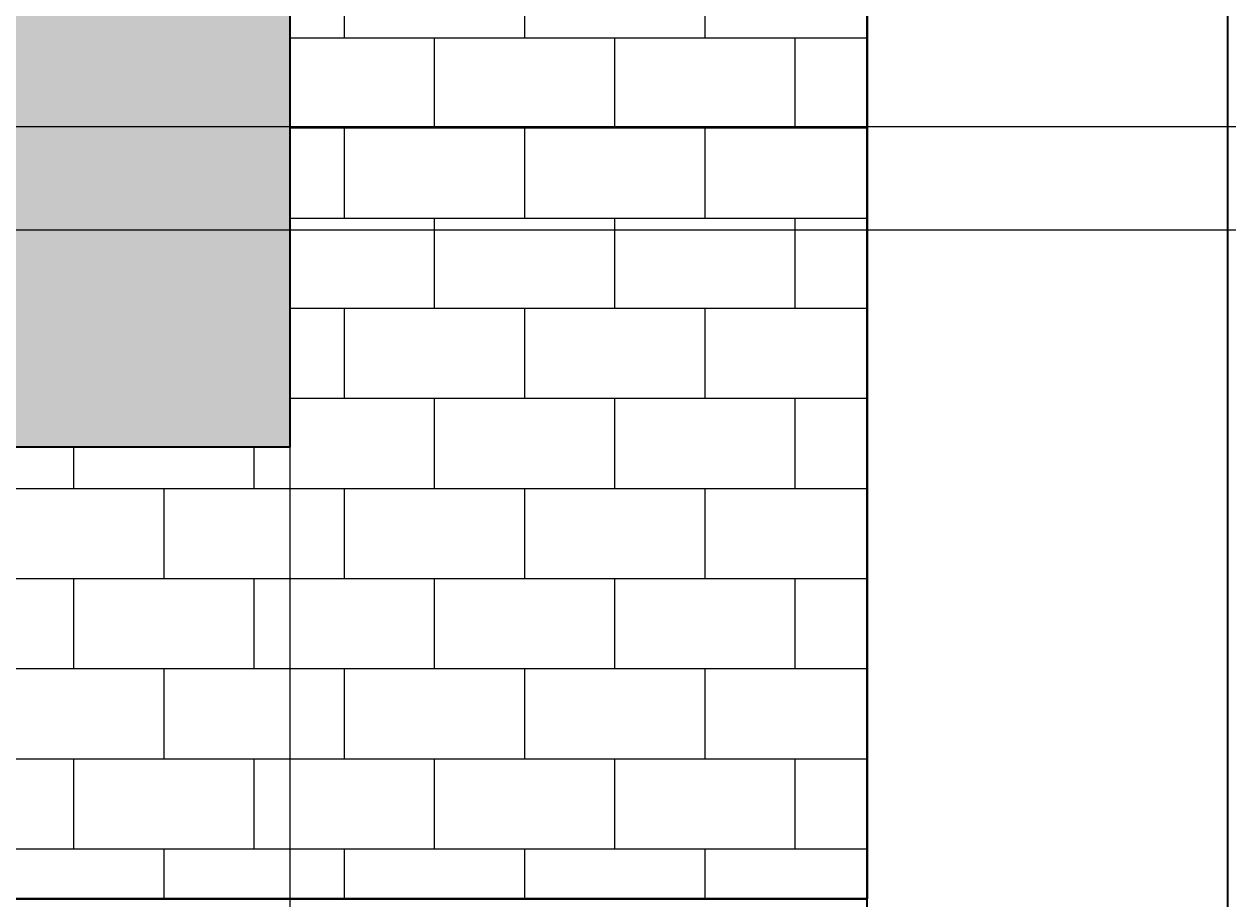
# Model space of a CAD drawing. Units: inches. Extents: x -13 to 809, y 112 to 656.
# Tile 46 of 55: x 521 to 621, y 251 to 324. Entities that reach past the tile are written whole.
import ezdxf

# ---------------------------------------------------------------- set-up
doc = ezdxf.new("R2010")
doc.units = ezdxf.units.IN
doc.header["$MEASUREMENT"] = 0
for name, color, linetype, lineweight in [('A-ANNO-DIMS', 2, 'Continuous', 18), ('A-ELEV', 7, 'Continuous', 35), ('A-ELEV-PATT', 8, 'Continuous', 13)]:
    doc.layers.add(name, color=color, linetype=linetype, lineweight=lineweight)
doc.styles.get("Standard").update_dxf_attribs({"font": 'arial.ttf'})
doc.dimstyles.get("Standard").update_dxf_attribs({"dimtxt": 0.625, "dimasz": 0.18, "dimexe": 0.18, "dimexo": 0.0625, "dimgap": 0.09, "dimtad": 0, "dimtih": 1, "dimtoh": 1, "dimdec": 4, "dimzin": 0, "dimdsep": 46, "dimlunit": 4, "dimtxsty": 'Standard', "dimcen": 0.09, "dimadec": 0, "dimazin": 0, "dimtfac": 1, "dimtdec": 4, "dimtofl": 0, "dimtmove": 0, "dimatfit": 3, "dimfxl": 1, "dimtolj": 1, "dimtzin": 0, "dimarcsym": 0})

# ---------------------------------------------------------------- blocks, each defined once
blk = doc.blocks.new('*D52')
at = {"layer": 'A-ANNO-DIMS', "color": 0, "lineweight": -2, "transparency": 16777216}
for p, q in [((442.18, 288.39), (442.18, 112.34)), ((542.96, 288.39), (542.96, 112.34)), ((442.36, 112.52), (491.21, 112.52)), ((542.78, 112.52), (493.93, 112.52))]:
    blk.add_line(p, q, dxfattribs=at)
at = {"layer": 'A-ANNO-DIMS', "color": 0, "transparency": 16777216}
for points in [[(442.36, 112.55), (442.36, 112.49), (442.18, 112.52)], [(542.78, 112.55), (542.78, 112.49), (542.96, 112.52)]]:
    blk.add_solid(points, dxfattribs=at)
at = {"layer": 'Defpoints', "color": 0, "transparency": 16777216}
for p in [(442.18, 288.45), (542.96, 288.45), (542.96, 112.52)]:
    blk.add_point(p, dxfattribs=at)
at = {"layer": 'A-ANNO-DIMS', "color": 0, "transparency": 16777216, "insert": (492.57, 112.52), "char_height": 0.625, "attachment_point": 5}
blk.add_mtext('\\A1;100.78', dxfattribs=at)
blk = doc.blocks.new('*D106')
at = {"layer": 'A-ANNO-DIMS', "color": 0, "lineweight": -2, "transparency": 16777216}
for p, q in [((319.57, 315.14), (807.77, 315.14)), ((807.59, 314.96), (807.59, 311.24)), ((807.59, 306.7), (807.59, 310.42)), ((337.57, 306.52), (807.77, 306.52))]:
    blk.add_line(p, q, dxfattribs=at)
at = {"layer": 'A-ANNO-DIMS', "color": 0, "transparency": 16777216}
for points in [[(807.56, 314.96), (807.62, 314.96), (807.59, 315.14)], [(807.56, 306.7), (807.62, 306.7), (807.59, 306.52)]]:
    blk.add_solid(points, dxfattribs=at)
at = {"layer": 'Defpoints', "color": 0, "transparency": 16777216}
for p in [(319.51, 315.14), (807.59, 315.14), (337.51, 306.52)]:
    blk.add_point(p, dxfattribs=at)
at = {"layer": 'A-ANNO-DIMS', "color": 0, "transparency": 16777216, "insert": (807.59, 310.83), "char_height": 0.625, "attachment_point": 5}
blk.add_mtext('\\A1;8.624', dxfattribs=at)

msp = doc.modelspace()

# ---------------------------------------------------------------- hatches: boundary and pattern name
at = {"layer": 'A-ELEV-PATT'}
h = msp.add_hatch(dxfattribs=at)
h.set_pattern_fill('BRICK', color=256, scale=30)
h.paths.add_polyline_path([(591.008, 558.5199), (341.4072, 558.5199), (341.4072, 524.281), (542.9617, 524.281), (542.9617, 288.4508), (341.4072, 288.4508), (341.4072, 250.8429), (591.008, 250.8429)])
h = msp.add_hatch(dxfattribs=at)
h.set_pattern_fill('CROSS', color=256, scale=9.7)
h.paths.add_polyline_path([(542.9617, 524.281), (442.1845, 524.281), (442.1845, 288.4508), (542.9617, 288.4508)])
h.paths.add_polyline_path([(471.0998, 470.8765), (471.0998, 498.1452), (510.462, 498.1452), (510.462, 470.8765)], flags=16)
h.paths.add_polyline_path([(473.0998, 472.8765), (473.0998, 496.1452), (508.462, 496.1452), (508.462, 472.8765)], flags=0)
h.paths.add_polyline_path([(471.0998, 442.128), (510.462, 442.128), (510.462, 414.8594), (471.0998, 414.8594)], flags=16)
h.paths.add_polyline_path([(473.0998, 440.128), (508.462, 440.128), (508.462, 416.8594), (473.0998, 416.8594)], flags=0)
h.paths.add_polyline_path([(471.0998, 385.2491), (510.462, 385.2491), (510.462, 357.9804), (471.0998, 357.9804)], flags=16)
h.paths.add_polyline_path([(473.0998, 383.2491), (508.462, 383.2491), (508.462, 359.9804), (473.0998, 359.9804)], flags=0)
h.paths.add_polyline_path([(471.0998, 340.4353), (510.462, 340.4353), (510.462, 313.1667), (471.0998, 313.1667)], flags=16)
h.paths.add_polyline_path([(473.0998, 338.4353), (508.462, 338.4353), (508.462, 315.1667), (473.0998, 315.1667)], flags=0)

# ---------------------------------------------------------------- linework, layer by layer
at = {"layer": 'A-ELEV'}
for p, q in [((591.008, 209.8635), (591.008, 558.5199)), ((621.008, 209.8635), (621.008, 558.5199)), ((341.4072, 250.8429), (591.008, 250.8429))]:
    msp.add_line(p, q, dxfattribs=at)
for points in [[(341.4072, 558.5199), (591.008, 558.5199), (591.008, 250.8429), (341.4072, 250.8429)], [(341.4072, 524.281), (542.9617, 524.281), (542.9617, 288.4508), (341.4072, 288.4508)]]:
    msp.add_lwpolyline(points, close=True, dxfattribs=at)

# ---------------------------------------------------------------- dimensions: what is measured, and where the dimension line sits
at = {"layer": 'A-ANNO-DIMS'}
dim = msp.add_linear_dim(base=(807.5888, 315.1435), p1=(337.5074, 306.5199), p2=(319.5074, 315.1435), angle=90, dimstyle='Standard', override={"dimdec": 3, "dimlfac": 1, "dimrnd": 0, "dimzin": 0, "dimdsep": 46, "dimlunit": 2}, dxfattribs=at)
dim.commit()
dim.dimension.update_dxf_attribs({"geometry": '*D106', "text_midpoint": (807.5888, 310.8317)})
dim = msp.add_linear_dim(base=(542.9617, 112.5199), p1=(442.1845, 288.4508), p2=(542.9617, 288.4508), dimstyle='Standard', override={"dimdec": 2, "dimlfac": 1, "dimrnd": 0, "dimzin": 0, "dimdsep": 46, "dimlunit": 2}, dxfattribs=at)
dim.commit()
dim.dimension.update_dxf_attribs({"geometry": '*D52', "text_midpoint": (492.5731, 112.5199)})

doc.saveas('drawing.dxf')
